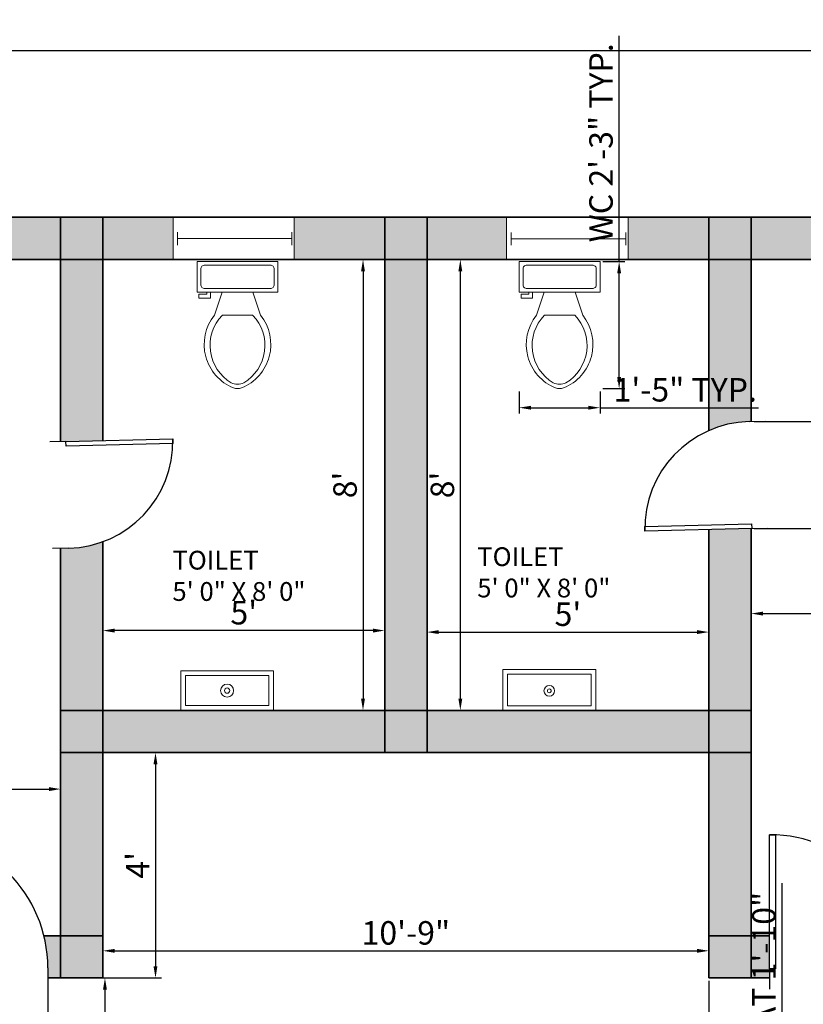
# Model space of a CAD drawing. Units: millimetres. Extents: x 2768 to 4359, y 795 to 1583.
# Tile 11 of 13: x 3764 to 3930, y 1373 to 1583. Entities that reach past the tile are written whole.
import ezdxf

# ---------------------------------------------------------------- set-up
doc = ezdxf.new("R2010")
doc.units = ezdxf.units.MM
for name, color, linetype, lineweight in [('A-ANNO-DIMS', 90, 'Continuous', 18), ('A-AREA-IDEN', 190, 'Continuous', 18), ('A-FLOR-FIXT', 50, 'Continuous', 18), ('A-WALL-PATT', 140, 'Continuous', 9), ('doors', 10, 'Continuous', 25), ('walls', 140, 'Continuous', 35), ('windows', 30, 'Continuous', 18)]:
    doc.layers.add(name, color=color, linetype=linetype, lineweight=lineweight)
doc.styles.get("Standard").update_dxf_attribs({"font": 'arial.ttf'})
doc.dimstyles.new('ISO-25', dxfattribs={"dimtxt": 5, "dimasz": 2.5, "dimexe": 1.25, "dimexo": 0.625, "dimtad": 1, "dimdec": 0, "dimlunit": 3, "dimtxsty": 'Standard', "dimcen": 2.5, "dimadec": 0, "dimazin": 0, "dimtfac": 1, "dimtdec": 0, "dimtmove": 0, "dimatfit": 3, "dimfxl": 1, "dimarcsym": 0})

# ---------------------------------------------------------------- blocks, each defined once
blk = doc.blocks.new('*U2')
for p, q in [((0, 0), (0, -6)), ((40, 0), (40, -6))]:
    blk.add_line(p, q)
blk.add_lwpolyline([(0, 0), (0, 40), (1.75, 40), (1.75, 0)], close=True)
blk.add_arc((0, 0), 40, 0, 90)
blk = doc.blocks.new('*U38')
for p, q in [((0, 4), (0, 0)), ((36, 4), (36, 0)), ((0, 2), (36, 2))]:
    blk.add_line(p, q)
blk = doc.blocks.new('Toilet - top')
for p, q in [((9.5, -6), (9.5, -2)), ((-10, -8.5), (-8, -8.5)), ((-10, -9.5), (-10, -8.5)), ((-7, -9.5), (-10, -9.5)), ((-8, -8.5), (-8, -8)), ((-7, -8), (-7, -9.5)), ((-4, -8), (-6, -14)), ((4, -8), (6, -14)), ((4, -14), (-4, -14))]:
    blk.add_line(p, q)
blk.add_lwpolyline([(10.5, -8), (10.5, 0), (-10.5, 0), (-10.5, -8)], close=True)
for points in [[(-9.5, -2), (-9.5, -6)], [(8.5, -1), (-8.5, -1)], [(-8.5, -7), (8.5, -7)]]:
    blk.add_lwpolyline(points)
for centre, radius, start, end in [((-8.62, -1.88), 0.884, 81.8699, 188.1301), ((8.62, -1.88), 0.884, 351.8699, 98.1301), ((-8.62, -6.12), 0.884, 171.8699, 278.1301), ((8.62, -6.12), 0.884, 261.8699, 8.1301), ((3.52, -21.58), 12.17, 141.4691, 247.9714), ((4.2, -21.82), 11.33, 136.3677, 238.9468), ((-3.52, -21.58), 12.17, 292.0284, 38.5307), ((-4.2, -21.82), 11.33, 301.053, 43.6321), ((0, -27.88), 4, 245.7318, 294.2682), ((0, -29), 4, 254.8605, 285.1395)]:
    blk.add_arc(centre, radius, start, end)
blk = doc.blocks.new('*D40')
at = {"layer": 'A-ANNO-DIMS', "color": 0, "lineweight": -2, "transparency": 16777216}
for p, q in [((3772.37, 1419.67), (3772.37, 1420.29)), ((3628.37, 1418.42), (3628.37, 1417.79)), ((3630.87, 1419.04), (3769.87, 1419.04))]:
    blk.add_line(p, q, dxfattribs=at)
at = {"layer": 'A-ANNO-DIMS', "color": 0, "transparency": 16777216}
for points in [[(3630.87, 1419.46), (3630.87, 1418.62), (3628.37, 1419.04)], [(3769.87, 1419.46), (3769.87, 1418.62), (3772.37, 1419.04)]]:
    blk.add_solid(points, dxfattribs=at)
at = {"layer": 'Defpoints', "color": 0, "transparency": 16777216}
for p in [(3628.37, 1419.04), (3772.37, 1419.04), (3772.37, 1419.04)]:
    blk.add_point(p, dxfattribs=at)
at = {"layer": 'A-ANNO-DIMS', "color": 0, "transparency": 16777216, "insert": (3700.37, 1422.18), "char_height": 5, "attachment_point": 5}
blk.add_mtext("12'", dxfattribs=at)
blk = doc.blocks.new('*D42')
at = {"layer": 'A-ANNO-DIMS', "color": 0, "lineweight": -2, "transparency": 16777216}
for p, q in [((3835.72, 1531.81), (3838, 1531.81)), ((3836.75, 1529.31), (3836.75, 1438.31)), ((3835.72, 1435.81), (3838, 1435.81))]:
    blk.add_line(p, q, dxfattribs=at)
at = {"layer": 'A-ANNO-DIMS', "color": 0, "transparency": 16777216}
for points in [[(3836.33, 1529.31), (3837.16, 1529.31), (3836.75, 1531.81)], [(3836.33, 1438.31), (3837.16, 1438.31), (3836.75, 1435.81)]]:
    blk.add_solid(points, dxfattribs=at)
at = {"layer": 'Defpoints', "color": 0, "transparency": 16777216}
for p in [(3835.1, 1531.81), (3835.1, 1435.81), (3836.75, 1435.81)]:
    blk.add_point(p, dxfattribs=at)
at = {"layer": 'A-ANNO-DIMS', "color": 0, "transparency": 16777216, "insert": (3833.57, 1483.81), "char_height": 5, "attachment_point": 5, "rotation": 90}
blk.add_mtext("8'", dxfattribs=at)
blk = doc.blocks.new('*D43')
at = {"layer": 'A-ANNO-DIMS', "color": 0, "lineweight": -2, "transparency": 16777216}
for p, q in [((3781.37, 1452.88), (3781.37, 1454.05)), ((3841.37, 1452.88), (3841.37, 1454.05)), ((3838.87, 1452.8), (3783.87, 1452.8))]:
    blk.add_line(p, q, dxfattribs=at)
at = {"layer": 'A-ANNO-DIMS', "color": 0, "transparency": 16777216}
for points in [[(3783.87, 1453.21), (3783.87, 1452.38), (3781.37, 1452.8)], [(3838.87, 1453.21), (3838.87, 1452.38), (3841.37, 1452.8)]]:
    blk.add_solid(points, dxfattribs=at)
at = {"layer": 'Defpoints', "color": 0, "transparency": 16777216}
for p in [(3781.37, 1452.8), (3781.37, 1452.26), (3841.37, 1452.26)]:
    blk.add_point(p, dxfattribs=at)
at = {"layer": 'A-ANNO-DIMS', "color": 0, "transparency": 16777216, "insert": (3811.37, 1455.96), "char_height": 5, "attachment_point": 5}
blk.add_mtext("5'", dxfattribs=at)
blk = doc.blocks.new('*D44')
at = {"layer": 'A-ANNO-DIMS', "color": 0, "lineweight": -2, "transparency": 16777216}
for p, q in [((3850.37, 1452.17), (3850.37, 1451.22)), ((3852.87, 1452.47), (3907.87, 1452.47)), ((3910.37, 1452.17), (3910.37, 1451.22))]:
    blk.add_line(p, q, dxfattribs=at)
at = {"layer": 'A-ANNO-DIMS', "color": 0, "transparency": 16777216}
for points in [[(3852.87, 1452.89), (3852.87, 1452.06), (3850.37, 1452.47)], [(3907.87, 1452.89), (3907.87, 1452.06), (3910.37, 1452.47)]]:
    blk.add_solid(points, dxfattribs=at)
at = {"layer": 'Defpoints', "color": 0, "transparency": 16777216}
for p in [(3850.37, 1452.8), (3910.37, 1452.8), (3910.37, 1452.47)]:
    blk.add_point(p, dxfattribs=at)
at = {"layer": 'A-ANNO-DIMS', "color": 0, "transparency": 16777216, "insert": (3880.37, 1455.64), "char_height": 5, "attachment_point": 5}
blk.add_mtext("5'", dxfattribs=at)
blk = doc.blocks.new('*D45')
at = {"layer": 'A-ANNO-DIMS', "color": 0, "lineweight": -2, "transparency": 16777216}
for p, q in [((3857.42, 1531.81), (3858.72, 1531.81)), ((3857.47, 1438.31), (3857.47, 1529.31)), ((3857.42, 1435.81), (3858.72, 1435.81))]:
    blk.add_line(p, q, dxfattribs=at)
at = {"layer": 'A-ANNO-DIMS', "color": 0, "transparency": 16777216}
for points in [[(3857.05, 1529.31), (3857.88, 1529.31), (3857.47, 1531.81)], [(3857.05, 1438.31), (3857.88, 1438.31), (3857.47, 1435.81)]]:
    blk.add_solid(points, dxfattribs=at)
at = {"layer": 'Defpoints', "color": 0, "transparency": 16777216}
for p in [(3856.8, 1531.81), (3857.47, 1531.81), (3856.8, 1435.81)]:
    blk.add_point(p, dxfattribs=at)
at = {"layer": 'A-ANNO-DIMS', "color": 0, "transparency": 16777216, "insert": (3854.29, 1483.81), "char_height": 5, "attachment_point": 5, "rotation": 90}
blk.add_mtext("8'", dxfattribs=at)
blk = doc.blocks.new('*D46')
at = {"layer": 'A-ANNO-DIMS', "color": 0, "lineweight": -2, "transparency": 16777216}
for p, q in [((3919.37, 1457.04), (3919.37, 1457.66)), ((4063.37, 1457.04), (4063.37, 1457.66)), ((3921.87, 1456.41), (4060.87, 1456.41))]:
    blk.add_line(p, q, dxfattribs=at)
at = {"layer": 'A-ANNO-DIMS', "color": 0, "transparency": 16777216}
for points in [[(3921.87, 1456.83), (3921.87, 1456), (3919.37, 1456.41)], [(4060.87, 1456.83), (4060.87, 1456), (4063.37, 1456.41)]]:
    blk.add_solid(points, dxfattribs=at)
at = {"layer": 'Defpoints', "color": 0, "transparency": 16777216}
for p in [(3919.37, 1456.41), (4063.37, 1456.41), (4063.37, 1456.41)]:
    blk.add_point(p, dxfattribs=at)
at = {"layer": 'A-ANNO-DIMS', "color": 0, "transparency": 16777216, "insert": (3991.37, 1459.55), "char_height": 5, "attachment_point": 5}
blk.add_mtext("12'", dxfattribs=at)
blk = doc.blocks.new('*D59')
at = {"layer": 'A-ANNO-DIMS', "color": 0, "lineweight": -2, "transparency": 16777216}
for p, q in [((3781.37, 1382.2), (3781.37, 1385.85)), ((3783.87, 1384.6), (3907.87, 1384.6)), ((3910.37, 1382.2), (3910.37, 1385.85))]:
    blk.add_line(p, q, dxfattribs=at)
at = {"layer": 'A-ANNO-DIMS', "color": 0, "transparency": 16777216}
for points in [[(3783.87, 1385.01), (3783.87, 1384.18), (3781.37, 1384.6)], [(3907.87, 1385.01), (3907.87, 1384.18), (3910.37, 1384.6)]]:
    blk.add_solid(points, dxfattribs=at)
at = {"layer": 'Defpoints', "color": 0, "transparency": 16777216}
for p in [(3910.37, 1384.6), (3781.37, 1381.58), (3910.37, 1381.58)]:
    blk.add_point(p, dxfattribs=at)
at = {"layer": 'A-ANNO-DIMS', "color": 0, "transparency": 16777216, "insert": (3845.87, 1387.77), "char_height": 5, "attachment_point": 5}
blk.add_mtext('10\'-9"', dxfattribs=at)
blk = doc.blocks.new('*D60')
at = {"layer": 'A-ANNO-DIMS', "color": 0, "lineweight": -2, "transparency": 16777216}
for p, q in [((3781.99, 1426.81), (3793.82, 1426.81)), ((3792.57, 1424.31), (3792.57, 1381.31)), ((3781.99, 1378.81), (3793.82, 1378.81))]:
    blk.add_line(p, q, dxfattribs=at)
at = {"layer": 'A-ANNO-DIMS', "color": 0, "transparency": 16777216}
for points in [[(3792.15, 1424.31), (3792.98, 1424.31), (3792.57, 1426.81)], [(3792.15, 1381.31), (3792.98, 1381.31), (3792.57, 1378.81)]]:
    blk.add_solid(points, dxfattribs=at)
at = {"layer": 'Defpoints', "color": 0, "transparency": 16777216}
for p in [(3781.37, 1426.81), (3781.37, 1378.81), (3792.57, 1378.81)]:
    blk.add_point(p, dxfattribs=at)
at = {"layer": 'A-ANNO-DIMS', "color": 0, "transparency": 16777216, "insert": (3789.44, 1402.81), "char_height": 5, "attachment_point": 5, "rotation": 90}
blk.add_mtext("4'", dxfattribs=at)
blk = doc.blocks.new('*D63')
at = {"layer": 'A-ANNO-DIMS', "color": 0, "lineweight": -2, "transparency": 16777216}
for p, q in [((3910.37, 1378.18), (3910.37, 1364.91)), ((3988.37, 1378.18), (3988.37, 1364.91)), ((3912.87, 1366.16), (3985.87, 1366.16))]:
    blk.add_line(p, q, dxfattribs=at)
at = {"layer": 'A-ANNO-DIMS', "color": 0, "transparency": 16777216}
for points in [[(3912.87, 1366.57), (3912.87, 1365.74), (3910.37, 1366.16)], [(3985.87, 1366.57), (3985.87, 1365.74), (3988.37, 1366.16)]]:
    blk.add_solid(points, dxfattribs=at)
at = {"layer": 'Defpoints', "color": 0, "transparency": 16777216}
for p in [(3910.37, 1378.81), (3988.37, 1378.81), (3988.37, 1366.16)]:
    blk.add_point(p, dxfattribs=at)
at = {"layer": 'A-ANNO-DIMS', "color": 0, "transparency": 16777216, "insert": (3949.37, 1369.33), "char_height": 5, "attachment_point": 5}
blk.add_mtext('6\'-6"', dxfattribs=at)
blk = doc.blocks.new('*D65')
at = {"layer": 'A-ANNO-DIMS', "color": 0, "lineweight": -2, "transparency": 16777216}
for p, q in [((3776.14, 1378.81), (3783.06, 1378.81)), ((3781.81, 1376.31), (3781.81, 1224.31)), ((3776.14, 1221.81), (3783.06, 1221.81))]:
    blk.add_line(p, q, dxfattribs=at)
at = {"layer": 'A-ANNO-DIMS', "color": 0, "transparency": 16777216}
for points in [[(3781.39, 1376.31), (3782.23, 1376.31), (3781.81, 1378.81)], [(3781.39, 1224.31), (3782.23, 1224.31), (3781.81, 1221.81)]]:
    blk.add_solid(points, dxfattribs=at)
at = {"layer": 'Defpoints', "color": 0, "transparency": 16777216}
for p in [(3775.51, 1378.81), (3775.51, 1221.81), (3781.81, 1221.81)]:
    blk.add_point(p, dxfattribs=at)
at = {"layer": 'A-ANNO-DIMS', "color": 0, "transparency": 16777216, "insert": (3778.63, 1300.31), "char_height": 5, "attachment_point": 5, "rotation": 90}
blk.add_mtext('13\'-1"', dxfattribs=at)
blk = doc.blocks.new('*D81')
at = {"layer": 'A-ANNO-DIMS', "color": 0, "lineweight": -2, "transparency": 16777216}
for p, q in [((3891.27, 1531.41), (3891.27, 1579.42)), ((3887.83, 1531.41), (3892.52, 1531.41)), ((3891.27, 1506.82), (3891.27, 1528.91)), ((3887.83, 1504.32), (3892.52, 1504.32))]:
    blk.add_line(p, q, dxfattribs=at)
at = {"layer": 'A-ANNO-DIMS', "color": 0, "transparency": 16777216}
for points in [[(3890.86, 1528.91), (3891.69, 1528.91), (3891.27, 1531.41)], [(3890.86, 1506.82), (3891.69, 1506.82), (3891.27, 1504.32)]]:
    blk.add_solid(points, dxfattribs=at)
at = {"layer": 'Defpoints', "color": 0, "transparency": 16777216}
for p in [(3887.21, 1531.41), (3891.27, 1531.41), (3887.21, 1504.32)]:
    blk.add_point(p, dxfattribs=at)
at = {"layer": 'A-ANNO-DIMS', "color": 0, "transparency": 16777216, "insert": (3888.06, 1556.67), "char_height": 5, "attachment_point": 5, "rotation": 90}
blk.add_mtext('WC 2\'-3" TYP.', dxfattribs=at)
blk = doc.blocks.new('*D82')
at = {"layer": 'A-ANNO-DIMS', "color": 0, "lineweight": -2, "transparency": 16777216}
for p, q in [((3869.99, 1503.7), (3869.99, 1499.01)), ((3887.21, 1503.7), (3887.21, 1499.01)), ((3872.49, 1500.26), (3884.71, 1500.26)), ((3887.21, 1500.26), (3920.97, 1500.26))]:
    blk.add_line(p, q, dxfattribs=at)
at = {"layer": 'A-ANNO-DIMS', "color": 0, "transparency": 16777216}
for points in [[(3872.49, 1500.67), (3872.49, 1499.84), (3869.99, 1500.26)], [(3884.71, 1500.67), (3884.71, 1499.84), (3887.21, 1500.26)]]:
    blk.add_solid(points, dxfattribs=at)
at = {"layer": 'Defpoints', "color": 0, "transparency": 16777216}
for p in [(3869.99, 1504.32), (3887.21, 1504.32), (3887.21, 1500.26)]:
    blk.add_point(p, dxfattribs=at)
at = {"layer": 'A-ANNO-DIMS', "color": 0, "transparency": 16777216, "insert": (3905.34, 1503.43), "char_height": 5, "attachment_point": 5}
blk.add_mtext('1\'-5" TYP.', dxfattribs=at)
blk = doc.blocks.new('*D111')
at = {"layer": 'A-ANNO-DIMS', "color": 0, "lineweight": -2, "transparency": 16777216}
for p, q in [((3925.95, 1339.44), (3925.95, 1398.97)), ((3923.3, 1339.44), (3927.2, 1339.44)), ((3925.95, 1320.11), (3925.95, 1336.94)), ((3923.3, 1317.61), (3927.2, 1317.61))]:
    blk.add_line(p, q, dxfattribs=at)
at = {"layer": 'A-ANNO-DIMS', "color": 0, "transparency": 16777216}
for points in [[(3925.53, 1336.94), (3926.37, 1336.94), (3925.95, 1339.44)], [(3925.53, 1320.11), (3926.37, 1320.11), (3925.95, 1317.61)]]:
    blk.add_solid(points, dxfattribs=at)
at = {"layer": 'Defpoints', "color": 0, "transparency": 16777216}
for p in [(3922.67, 1339.44), (3925.95, 1339.44), (3922.67, 1317.61)]:
    blk.add_point(p, dxfattribs=at)
at = {"layer": 'A-ANNO-DIMS', "color": 0, "transparency": 16777216, "insert": (3922.74, 1370.46), "char_height": 5, "attachment_point": 5, "rotation": 90}
blk.add_mtext('LOVESEAT 1\'-10"', dxfattribs=at)
blk = doc.blocks.new('*D128')
at = {"layer": 'A-ANNO-DIMS', "color": 0, "lineweight": -2, "transparency": 16777216}
for p, q in [((3619.37, 1541.43), (3619.37, 1577.56)), ((4322.37, 1541.43), (4322.37, 1577.56)), ((3621.87, 1576.31), (4319.87, 1576.31))]:
    blk.add_line(p, q, dxfattribs=at)
at = {"layer": 'A-ANNO-DIMS', "color": 0, "transparency": 16777216}
for points in [[(3621.87, 1576.72), (3621.87, 1575.89), (3619.37, 1576.31)], [(4319.87, 1576.72), (4319.87, 1575.89), (4322.37, 1576.31)]]:
    blk.add_solid(points, dxfattribs=at)
at = {"layer": 'Defpoints', "color": 0, "transparency": 16777216}
for p in [(4322.37, 1576.31), (3619.37, 1540.81), (4322.37, 1540.81)]:
    blk.add_point(p, dxfattribs=at)
at = {"layer": 'A-ANNO-DIMS', "color": 0, "transparency": 16777216, "insert": (3970.87, 1579.49), "char_height": 5, "attachment_point": 5}
blk.add_mtext('58\'-7"', dxfattribs=at)
blk = doc.blocks.new('*D135')
at = {"layer": 'A-ANNO-DIMS', "color": 0, "lineweight": -2, "transparency": 16777216}
for p, q in [((3741.08, 1378.18), (3741.08, 798.41)), ((3769.66, 1378.18), (3769.66, 798.41)), ((3743.58, 799.66), (3767.16, 799.66))]:
    blk.add_line(p, q, dxfattribs=at)
at = {"layer": 'A-ANNO-DIMS', "color": 0, "transparency": 16777216}
for points in [[(3743.58, 800.08), (3743.58, 799.24), (3741.08, 799.66)], [(3767.16, 800.08), (3767.16, 799.24), (3769.66, 799.66)]]:
    blk.add_solid(points, dxfattribs=at)
at = {"layer": 'Defpoints', "color": 0, "transparency": 16777216}
for p in [(3741.08, 1378.81), (3769.66, 1378.81), (3769.66, 799.66)]:
    blk.add_point(p, dxfattribs=at)
at = {"layer": 'A-ANNO-DIMS', "color": 0, "transparency": 16777216, "insert": (3755.37, 802.87), "char_height": 5, "attachment_point": 5}
blk.add_mtext('2\'-4 1/2"', dxfattribs=at)
blk = doc.blocks.new('*D136')
at = {"layer": 'A-ANNO-DIMS', "color": 0, "lineweight": -2, "transparency": 16777216}
for p, q in [((3919.99, 1497.31), (4359.12, 1497.31)), ((4357.87, 1477.05), (4357.87, 1494.81)), ((3919.99, 1474.55), (4359.12, 1474.55))]:
    blk.add_line(p, q, dxfattribs=at)
at = {"layer": 'A-ANNO-DIMS', "color": 0, "transparency": 16777216}
for points in [[(4357.45, 1494.81), (4358.28, 1494.81), (4357.87, 1497.31)], [(4357.45, 1477.05), (4358.28, 1477.05), (4357.87, 1474.55)]]:
    blk.add_solid(points, dxfattribs=at)
at = {"layer": 'Defpoints', "color": 0, "transparency": 16777216}
for p in [(3919.37, 1497.31), (4357.87, 1497.31), (3919.37, 1474.55)]:
    blk.add_point(p, dxfattribs=at)
at = {"layer": 'A-ANNO-DIMS', "color": 0, "transparency": 16777216, "insert": (4354.73, 1485.93), "char_height": 5, "attachment_point": 5, "rotation": 90}
blk.add_mtext('1\'-11"', dxfattribs=at)

msp = doc.modelspace()

# ---------------------------------------------------------------- hatches: boundary and pattern name
at = {"layer": 'A-WALL-PATT'}
h = msp.add_hatch(color=256, dxfattribs=at)
h.dxf.hatch_style = 1
h.paths.add_polyline_path([(3666.8, 1540.81), (3628.37, 1540.81), (3628.37, 1531.81), (3666.8, 1531.81)])
h.paths.add_polyline_path([(3628.37, 1540.81), (3619.37, 1540.81), (3619.37, 1531.81), (3628.37, 1531.81)])
h.paths.add_polyline_path([(3628.37, 1531.81), (3619.37, 1531.81), (3619.37, 1387.81), (3628.37, 1387.81)])
h.paths.add_polyline_path([(3772.37, 1540.81), (3710.62, 1540.81), (3710.62, 1531.81), (3772.37, 1531.81)])
h.paths.add_polyline_path([(3796.31, 1540.81), (3781.37, 1540.81), (3781.37, 1531.81), (3796.31, 1531.81)])
h.paths.add_polyline_path([(3781.37, 1540.81), (3772.37, 1540.81), (3772.37, 1531.81), (3781.37, 1531.81)])
h.paths.add_polyline_path([(3781.37, 1531.81), (3772.37, 1531.81), (3772.37, 1493.05), (3773.51, 1493.08), (3781.37, 1493.27)])
h.paths.add_polyline_path([(3841.37, 1540.81), (3822.12, 1540.81), (3822.12, 1531.81), (3841.37, 1531.81)])
h.paths.add_polyline_path([(3867.29, 1540.81), (3850.37, 1540.81), (3850.37, 1531.81), (3867.29, 1531.81)])
h.paths.add_polyline_path([(3850.37, 1540.81), (3841.37, 1540.81), (3841.37, 1531.81), (3850.37, 1531.81)])
h.paths.add_polyline_path([(3850.37, 1531.81), (3841.37, 1531.81), (3841.37, 1435.81), (3850.37, 1435.81)])
h.paths.add_polyline_path([(3919.37, 1531.81), (3910.37, 1531.81), (3910.37, 1495.39, -0.097322), (3918.93, 1497.3), (3919.37, 1497.31)])
h.paths.add_polyline_path([(3919.37, 1540.81), (3910.37, 1540.81), (3910.37, 1531.81), (3919.37, 1531.81)])
h.paths.add_polyline_path([(3910.37, 1540.81), (3893.19, 1540.81), (3893.19, 1531.81), (3910.37, 1531.81)])
h.paths.add_polyline_path([(3971.85, 1540.81), (3919.37, 1540.81), (3919.37, 1531.81), (3971.85, 1531.81)])
h.paths.add_polyline_path([(4063.37, 1540.81), (4017.44, 1540.81), (4017.44, 1531.81), (4063.37, 1531.81)])
h.paths.add_polyline_path([(4072.37, 1531.81), (4063.37, 1531.81), (4063.37, 1387.81), (4072.37, 1387.81)])
h.paths.add_polyline_path([(4072.37, 1378.81), (4063.37, 1378.81), (4063.37, 1240.81), (4072.37, 1240.81)])
h.paths.add_polyline_path([(4072.37, 1387.81), (4063.37, 1387.81), (4063.37, 1378.81), (4072.37, 1378.81)])
h.paths.add_polyline_path([(3919.37, 1387.81), (3910.37, 1387.81), (3910.37, 1378.81), (3919.37, 1378.81)])
h.paths.add_polyline_path([(3919.37, 1392.95, -0.05459), (3913.18, 1392.28), (3910.37, 1392.28), (3910.37, 1387.81), (3919.37, 1387.81)])
h.paths.add_polyline_path([(3919.37, 1474.55), (3910.37, 1474.32), (3910.37, 1435.81), (3919.37, 1435.81)])
h.paths.add_polyline_path([(3919.37, 1435.81), (3910.37, 1435.81), (3910.37, 1426.81), (3919.37, 1426.81)])
h.paths.add_polyline_path([(3910.37, 1435.81), (3850.37, 1435.81), (3850.37, 1426.81), (3910.37, 1426.81)])
h.paths.add_polyline_path([(3919.37, 1426.81), (3910.37, 1426.81), (3910.37, 1420.86), (3913.18, 1420.86), (3919.37, 1420.86)])
h.paths.add_polyline_path([(3850.37, 1435.81), (3841.37, 1435.81), (3841.37, 1426.81), (3850.37, 1426.81)])
h.paths.add_polyline_path([(3841.37, 1435.81), (3781.37, 1435.81), (3781.37, 1426.81), (3841.37, 1426.81)])
h.paths.add_polyline_path([(3781.37, 1435.81), (3772.37, 1435.81), (3772.37, 1426.81), (3781.37, 1426.81)])
h.paths.add_polyline_path([(3781.37, 1426.81), (3772.37, 1426.81), (3772.37, 1420.59, -0.050492), (3778.09, 1421.17), (3781.37, 1421.17)])
h.paths.add_polyline_path([(3781.37, 1471.72, -0.082137), (3774.07, 1470.33), (3772.37, 1470.29), (3772.37, 1435.81), (3781.37, 1435.81)])
h.paths.add_polyline_path([(3628.37, 1387.81), (3619.37, 1387.81), (3619.37, 1378.81), (3628.37, 1378.81)])
h.paths.add_polyline_path([(3628.37, 1378.81), (3619.37, 1378.81), (3619.37, 1346.39), (3622.95, 1346.39), (3628.37, 1346.39)])
h.paths.add_polyline_path([(3781.37, 1387.81), (3772.37, 1387.81), (3772.37, 1378.81), (3781.37, 1378.81)])
h.paths.add_polyline_path([(3781.37, 1392.59), (3778.09, 1392.59), (3772.37, 1392.59), (3772.37, 1387.81), (3781.37, 1387.81)])
h.paths.add_polyline_path([(3628.37, 1318.32, -0.047705), (3622.95, 1317.81), (3619.37, 1317.81), (3619.37, 1221.81), (3628.37, 1221.81)])
h.paths.add_polyline_path([(3628.37, 1221.81), (3619.37, 1221.81), (3619.37, 1212.81), (3628.37, 1212.81)])
h.paths.add_polyline_path([(3827.37, 1221.81), (3628.37, 1221.81), (3628.37, 1212.81), (3827.37, 1212.81)])
h.paths.add_polyline_path([(3628.37, 1212.81), (3619.37, 1212.81), (3619.37, 1116.81), (3628.37, 1116.81)])
h.paths.add_polyline_path([(3836.37, 1221.81), (3827.37, 1221.81), (3827.37, 1212.81), (3836.37, 1212.81)])
h.paths.add_polyline_path([(3628.37, 1107.81), (3619.37, 1107.81), (3619.37, 1047.81), (3628.37, 1047.81)])
h.paths.add_polyline_path([(3628.37, 1116.81), (3619.37, 1116.81), (3619.37, 1107.81), (3628.37, 1107.81)])
h.paths.add_polyline_path([(3836.37, 1155.81), (3827.37, 1155.81), (3827.37, 1116.81), (3836.37, 1116.81)])
h.paths.add_polyline_path([(3836.37, 1116.81), (3827.37, 1116.81), (3827.37, 1107.81), (3836.37, 1107.81)])
h.paths.add_polyline_path([(3836.37, 1107.81), (3827.37, 1107.81), (3827.37, 1047.81), (3836.37, 1047.81)])
h.paths.add_polyline_path([(3827.37, 1047.37), (3827.37, 1047.81), (3739.96, 1047.81), (3739.96, 1038.81), (3827.37, 1038.81)])
h.paths.add_polyline_path([(3836.37, 1047.37), (3836.37, 1047.81), (3827.37, 1047.81), (3827.37, 1047.37), (3827.37, 1038.81), (3836.37, 1038.81)])
h.paths.add_polyline_path([(3695.08, 1047.81), (3628.37, 1047.81), (3628.37, 1038.81), (3695.08, 1038.81)])
h.paths.add_polyline_path([(3628.37, 1047.81), (3619.37, 1047.81), (3619.37, 1038.81), (3628.37, 1038.81)])
h.paths.add_polyline_path([(3850.59, 1047.81), (3836.37, 1047.81), (3836.37, 1047.37), (3836.37, 1038.81), (3850.59, 1038.81)])
h.paths.add_polyline_path([(3896.37, 1047.37), (3896.37, 1047.81), (3876.26, 1047.81), (3876.26, 1038.81), (3896.37, 1038.81)])
h.paths.add_polyline_path([(3905.37, 1109.65), (3903.46, 1109.6), (3896.37, 1109.43), (3896.37, 1047.81), (3905.37, 1047.81)])
h.paths.add_polyline_path([(3905.37, 1047.81), (3896.37, 1047.81), (3896.37, 1047.37), (3896.37, 1038.81), (3905.37, 1038.81)])
h.paths.add_polyline_path([(4063.37, 1047.81), (3905.37, 1047.81), (3905.37, 1038.81), (4063.37, 1038.81)])
h.paths.add_polyline_path([(4072.37, 1137.28), (4063.37, 1137.28), (4063.37, 1047.81), (4072.37, 1047.81)])
h.paths.add_polyline_path([(4072.37, 1231.81), (4063.37, 1231.81), (4063.37, 1182.55), (4072.37, 1182.55)])
h.paths.add_polyline_path([(4072.37, 1240.81), (4063.37, 1240.81), (4063.37, 1231.81), (4072.37, 1231.81)])
h.paths.add_polyline_path([(4072.37, 1047.81), (4063.37, 1047.81), (4063.37, 1038.81), (4072.37, 1038.81)])
h.paths.add_polyline_path([(3905.37, 1231.81), (3896.37, 1231.81), (3896.37, 1164.81), (3905.37, 1164.81)])
h.paths.add_polyline_path([(3905.37, 1240.81), (3896.37, 1240.81), (3896.37, 1231.81), (3905.37, 1231.81)])
h.paths.add_polyline_path([(3910.61, 1237.57), (3910.61, 1240.81), (3905.37, 1240.81), (3905.37, 1231.81), (3911.2, 1231.81, -0.050754)])
h.paths.add_polyline_path([(3988.37, 1240.81), (3939.19, 1240.81), (3939.19, 1237.57), (3939.19, 1231.81), (3988.37, 1231.81)])
h.paths.add_polyline_path([(3997.37, 1240.81), (3988.37, 1240.81), (3988.37, 1231.81), (3997.37, 1231.81)])
h.paths.add_polyline_path([(4063.37, 1240.81), (3997.37, 1240.81), (3997.37, 1231.81), (4063.37, 1231.81)])
h.paths.add_polyline_path([(3997.37, 1334.21), (3988.37, 1334.21), (3988.37, 1288.44), (3997.37, 1288.44)])
h.paths.add_polyline_path([(3896.37, 1164.81), (3836.37, 1164.81), (3836.37, 1155.81), (3896.37, 1155.81)])
h.paths.add_polyline_path([(3836.37, 1164.81), (3827.37, 1164.81), (3827.37, 1155.81), (3836.37, 1155.81)])
h.paths.add_polyline_path([(3905.37, 1164.81), (3896.37, 1164.81), (3896.37, 1155.81), (3905.37, 1155.81)])
h.paths.add_polyline_path([(3905.37, 1155.81), (3896.37, 1155.81), (3896.37, 1131.22, -0.073168), (3902.89, 1132.35), (3905.37, 1132.41)])
edge = h.paths.add_edge_path()
edge.add_line((3951.89, 1380.74), (3951.89, 1378.81))
edge.add_line((3951.89, 1378.81), (4063.37, 1378.81))
edge.add_line((4063.37, 1378.81), (4063.37, 1387.81))
edge.add_line((4063.37, 1387.81), (3951, 1387.81))
edge.add_arc((3923.31, 1380.74), 28.58, 0, 14.3236, ccw=False)
h.paths.add_polyline_path([(3923.31, 1378.81), (3923.31, 1387.81), (3919.37, 1387.81), (3919.37, 1378.81)])
edge = h.paths.add_edge_path()
edge.add_arc((3775.74, 1114.53), 22.75, 187.4686, 197.1843)
edge.add_line((3754, 1107.81), (3628.37, 1107.81))
edge.add_line((3628.37, 1107.81), (3628.37, 1116.81))
edge.add_line((3628.37, 1116.81), (3752.42, 1116.81))
edge.add_arc((3775.17, 1117.41), 22.75, 181.5276, 194.8757)
h.paths.add_polyline_path([(3775.68, 1116.81), (3775.91, 1107.81), (3827.37, 1107.81), (3827.37, 1116.81)])
h = msp.add_hatch(color=256, dxfattribs=at)
h.dxf.hatch_style = 1
h.paths.add_polyline_path([(3781.37, 1426.81), (3772.37, 1426.81), (3772.37, 1387.81), (3781.37, 1387.81), (3781.37, 1392.59)])
h.paths.add_polyline_path([(3919.37, 1426.81), (3910.37, 1426.81), (3910.37, 1387.81), (3919.37, 1387.81)])
h = msp.add_hatch(color=256, dxfattribs=at)
h.dxf.hatch_style = 1
h.paths.add_polyline_path([(3628.37, 1387.81), (3628.37, 1378.81), (3741.08, 1378.81), (3741.08, 1380.94), (3741.08, 1387.81)])
h.paths.add_polyline_path([(3769.66, 1380.94), (3769.66, 1378.81), (3772.37, 1378.81), (3772.37, 1387.81), (3768.82, 1387.81, -0.060722)])

# ---------------------------------------------------------------- linework, layer by layer
at = {"layer": 'A-FLOR-FIXT'}
for points in [[(3797.96, 1435.81), (3817.67, 1435.81), (3817.67, 1444.22), (3797.96, 1444.22)], [(3798.96, 1436.81), (3816.67, 1436.81), (3816.67, 1443.22), (3798.96, 1443.22)], [(3866.49, 1435.79), (3886.31, 1435.79), (3886.31, 1444.51), (3866.49, 1444.51)], [(3867.49, 1436.79), (3885.31, 1436.79), (3885.31, 1443.51), (3867.49, 1443.51)]]:
    msp.add_lwpolyline(points, close=True, dxfattribs=at)
for centre, radius in [((3807.82, 1440.01), 1.39), ((3807.82, 1440.01), 0.562), ((3876.4, 1439.97), 1.14), ((3876.4, 1439.97), 0.411)]:
    msp.add_circle(centre, radius, dxfattribs=at)
at = {"layer": 'walls'}
for p, q in [((3619.37, 1540.81), (4322.37, 1540.81)), ((3772.37, 1540.81), (3772.37, 1493.05)), ((3781.37, 1540.81), (3781.37, 1493.27)), ((3841.37, 1540.81), (3841.37, 1426.81)), ((3850.37, 1540.81), (3850.37, 1426.81)), ((3910.37, 1540.81), (3910.37, 1495.39)), ((3919.37, 1540.81), (3919.37, 1497.31)), ((3619.37, 1531.81), (4322.37, 1531.81)), ((3910.37, 1474.32), (3910.37, 1387.81)), ((3919.37, 1474.55), (3919.37, 1387.81)), ((3772.37, 1470.29), (3772.37, 1387.81)), ((3781.37, 1471.72), (3781.37, 1387.81)), ((3772.37, 1435.81), (3919.37, 1435.81)), ((3772.37, 1426.81), (3919.37, 1426.81)), ((3772.37, 1392.59), (3772.37, 1378.81)), ((3781.37, 1392.59), (3781.37, 1378.81)), ((3919.37, 1392.95), (3919.37, 1378.81)), ((3910.37, 1392.28), (3910.37, 1378.81)), ((3768.82, 1387.81), (3781.37, 1387.81)), ((3768.82, 1387.81), (3781.37, 1387.81)), ((3910.37, 1387.81), (3923.31, 1387.81)), ((3769.66, 1378.81), (3781.37, 1378.81)), ((3769.66, 1378.81), (3781.37, 1378.81)), ((3910.37, 1378.81), (3923.31, 1378.81))]:
    msp.add_line(p, q, dxfattribs=at)
at = {"layer": 'windows'}
for p, q in [((3796.31, 1540.81), (3796.31, 1531.81)), ((3822.12, 1540.81), (3822.12, 1531.81)), ((3867.29, 1540.81), (3867.29, 1531.81)), ((3893.19, 1540.81), (3893.19, 1531.81))]:
    msp.add_line(p, q, dxfattribs=at)

# ---------------------------------------------------------------- block references
at = {"layer": 'A-FLOR-FIXT', "xscale": 0.8198293792319322, "yscale": 0.8198293792319322, "zscale": 0.8198293792319322}
for p in [(3810.03, 1531.41), (3878.6, 1531.41)]:
    msp.add_blockref('Toilet - top', p, dxfattribs=at)
at = {"layer": 'doors', "xscale": 0.5688608536322607, "yscale": 0.5688608536322607, "zscale": 0.5688608536322607}
for p, rotation in [((3919.5, 1474.55), 91.42344245075623), ((3773.51, 1493.08), 271.4234424507562)]:
    msp.add_blockref('*U2', p, dxfattribs=dict(at, rotation=rotation))
at = {"layer": 'doors', "xscale": 0.7144929449846577, "yscale": 0.7144929449846577, "zscale": 0.7144929449846577}
for p in [(3741.08, 1380.94), (3923.31, 1380.74)]:
    msp.add_blockref('*U2', p, dxfattribs=at)
at = {"layer": 'windows', "xscale": 0.6767405614116047, "yscale": 0.6767405614116047, "zscale": 0.6767405614116047}
for p in [(3797.22, 1534.91), (3868.31, 1534.85)]:
    msp.add_blockref('*U38', p, dxfattribs=at)

# ---------------------------------------------------------------- texts
at = {"layer": 'A-AREA-IDEN', "char_height": 4, "attachment_point": 1}
for width, insert in [(29.0411, (3861.07, 1470.53)), (34.3714, (3796.17, 1469.79))]:
    msp.add_mtext_dynamic_manual_height_columns('TOILET \\P5\' 0" X 8\' 0"', width=width, gutter_width=12.5, heights=[0], dxfattribs=dict(at, insert=insert))

# ---------------------------------------------------------------- dimensions: what is measured, and where the dimension line sits
at = {"layer": 'A-ANNO-DIMS'}
for base, p1, p2, override, picture, middle in [((4322.37, 1576.31), (3619.37, 1540.81), (4322.37, 1540.81), {"dimdec": 1, "dimlfac": 1, "dimrnd": 0, "dimzin": 1, "dimdsep": 46, "dimlunit": 4, "dimfrac": 2}, '*D128', (3970.87, 1579.49)), ((4063.37, 1456.41), (3919.37, 1456.41), (4063.37, 1456.41), {"dimclrd": 0, "dimclre": 0, "dimclrt": 0}, '*D46', (3991.37, 1459.55)), ((3781.37, 1452.8), (3841.37, 1452.26), (3781.37, 1452.26), {"dimclrd": 0, "dimclre": 0, "dimclrt": 0}, '*D43', (3811.37, 1455.96)), ((3910.37, 1452.47), (3850.37, 1452.8), (3910.37, 1452.8), {"dimclrd": 0, "dimclre": 0, "dimclrt": 0}, '*D44', (3880.37, 1455.64)), ((3772.37, 1419.04), (3628.37, 1419.04), (3772.37, 1419.04), {"dimclrd": 0, "dimclre": 0, "dimclrt": 0}, '*D40', (3700.37, 1422.18)), ((3910.37, 1384.6), (3781.37, 1381.58), (3910.37, 1381.58), {"dimclrd": 0, "dimclre": 0, "dimclrt": 0}, '*D59', (3845.87, 1387.77)), ((3769.66, 799.66), (3741.08, 1378.81), (3769.66, 1378.81), {"dimdec": 1, "dimlfac": 1, "dimrnd": 0, "dimzin": 1, "dimdsep": 46, "dimlunit": 4, "dimfrac": 2}, '*D135', (3755.37, 802.87)), ((3988.37, 1366.16), (3910.37, 1378.81), (3988.37, 1378.81), {"dimclrd": 0, "dimclre": 0, "dimclrt": 0}, '*D63', (3949.37, 1369.33))]:
    dim = msp.add_linear_dim(base=base, p1=p1, p2=p2, dimstyle='ISO-25', override=override, dxfattribs=at)
    dim.commit()
    dim.dimension.update_dxf_attribs({"geometry": picture, "text_midpoint": middle})
for base, p1, p2, text, picture, middle in [((3891.27, 1531.41), (3887.21, 1504.32), (3887.21, 1531.41), 'WC <> TYP.', '*D81', (3888.06, 1556.67)), ((3925.95, 1339.44), (3922.67, 1317.61), (3922.67, 1339.44), 'LOVESEAT <>', '*D111', (3922.74, 1370.46))]:
    dim = msp.add_linear_dim(base=base, p1=p1, p2=p2, angle=90, text=text, dimstyle='ISO-25', override={"dimdec": 1, "dimlfac": 1, "dimrnd": 0, "dimzin": 1, "dimdsep": 46, "dimlunit": 4, "dimfrac": 2}, dxfattribs=at)
    dim.commit()
    dim.dimension.update_dxf_attribs({"geometry": picture, "text_midpoint": middle})
for base, p1, p2, override, picture, middle in [((3836.75, 1435.81), (3835.1, 1531.81), (3835.1, 1435.81), {"dimclrd": 0, "dimclre": 0, "dimclrt": 0}, '*D42', (3833.57, 1483.81)), ((3857.47, 1531.81), (3856.8, 1435.81), (3856.8, 1531.81), {"dimclrd": 0, "dimclre": 0, "dimclrt": 0}, '*D45', (3854.29, 1483.81)), ((4357.87, 1497.31), (3919.37, 1474.55), (3919.37, 1497.31), {"dimdec": 1, "dimlfac": 1, "dimrnd": 0, "dimzin": 1, "dimdsep": 46, "dimlunit": 4, "dimfrac": 2}, '*D136', (4354.73, 1485.93)), ((3792.57, 1378.81), (3781.37, 1426.81), (3781.37, 1378.81), {"dimclrd": 0, "dimclre": 0, "dimclrt": 0}, '*D60', (3789.44, 1402.81)), ((3781.81, 1221.81), (3775.51, 1378.81), (3775.51, 1221.81), {"dimclrd": 0, "dimclre": 0, "dimclrt": 0}, '*D65', (3778.63, 1300.31))]:
    dim = msp.add_linear_dim(base=base, p1=p1, p2=p2, angle=90, dimstyle='ISO-25', override=override, dxfattribs=at)
    dim.commit()
    dim.dimension.update_dxf_attribs({"geometry": picture, "text_midpoint": middle})
dim = msp.add_linear_dim(base=(3887.21, 1500.26), p1=(3869.99, 1504.32), p2=(3887.21, 1504.32), text='<> TYP.', dimstyle='ISO-25', override={"dimdec": 1, "dimlfac": 1, "dimrnd": 0, "dimzin": 1, "dimdsep": 46, "dimlunit": 4, "dimfrac": 2}, dxfattribs=at)
dim.commit()
dim.dimension.update_dxf_attribs({"geometry": '*D82', "text_midpoint": (3905.34, 1503.43)})

doc.saveas('drawing.dxf')
